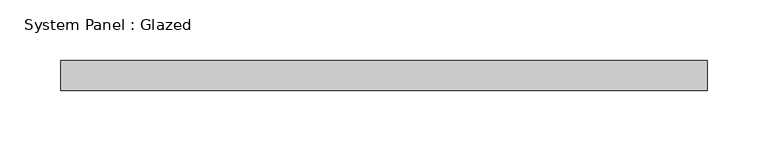
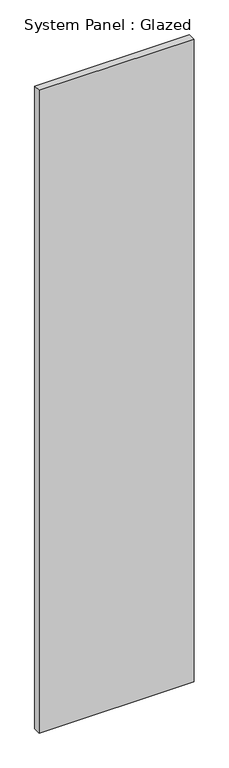
"""IFC4 building model written with IfcOpenShell, lengths in millimetres: plate geometry, System Panel : Glazed."""

from ifc_helpers import new_model, si_unit, origin, origin_with_axes, place, context, project, spatial, polyline, outline, extrude, source, transform, mapped, element, save


def system_panel_glazed_90abe38c(model_context):
    return source(origin(), model_context, "Body", "SweptSolid", [
        extrude(outline(polyline([(266.7, 24.5), (-266.7, 24.5), (-266.7, 49.5), (266.7, 49.5), (266.7, 24.5)])), origin_with_axes(), (0.0, 0.0, 1.0), 2338.4),
    ])


if __name__ == "__main__":
    model = new_model("IFC4")
    model_context = context("Model", 3, world=origin())
    ifc_project = project(units=[si_unit("LENGTHUNIT", "METRE", prefix="MILLI")], contexts=[model_context])
    site = spatial("IfcSite", under=ifc_project)
    building = spatial("IfcBuilding", under=site)
    placement = place(None, origin())
    system_panel_glazed_shape = system_panel_glazed_90abe38c(model_context)
    element("IfcPlate", 1, ObjectType="System Panel : Glazed", at=placement, inside=building, context=model_context, shape_type="MappedRepresentation", body=[
        mapped(system_panel_glazed_shape, transform((0.0, 0.0, 0.0), x_axis=(1.0, 0.0, 0.0), y_axis=(0.0, 1.0, 0.0), z_axis=(0.0, 0.0, 1.0))),
    ])
    save(model, "model.ifc")

# Revit data of these elements
# Type "System Panel : Glazed"
#   Construction Type Id = "GSP4R"
#   Analytic Construction = "1/8 in Pilkington single glazing"
#   Visual Light Transmittance = 0.9
#   Solar Heat Gain Coefficient = 0.86
#   Heat Transfer Coefficient (U) = 6.7069 W/(m²·K)
# Element 1 (IfcPlate, "System Panel : Glazed")
#   Materials on its faces: "Glass"
# Materials
#   "Glass": class "Glass", colour RGB 0 128 192, transparency 0.9, Description = "Soda Lime Glass", Cost = 0
